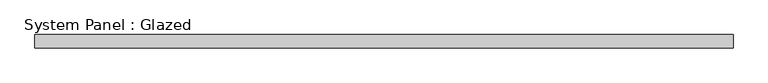
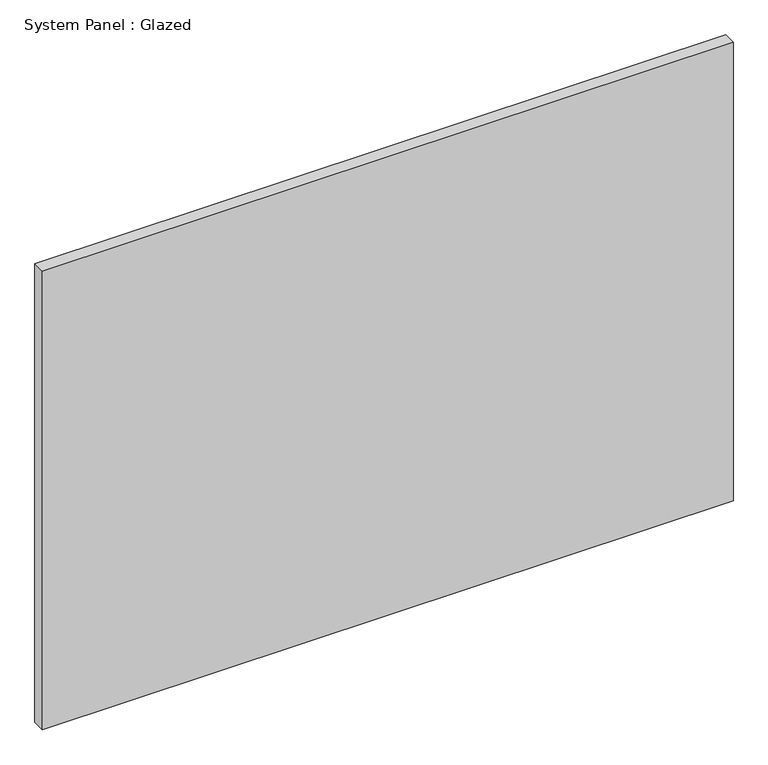
"""IFC4 building model written with IfcOpenShell, lengths in millimetres: plate geometry, System Panel : Glazed."""

from ifc_helpers import new_model, si_unit, origin, origin_with_axes, place, context, project, spatial, polyline, outline, extrude, source, transform, mapped, element, save


def system_panel_glazed_dc01897a(model_context):
    return source(origin(), model_context, "Body", "SweptSolid", [
        extrude(outline(polyline([(660.8, 24.5), (-660.8, 24.5), (-660.8, 49.5), (660.8, 49.5), (660.8, 24.5)])), origin_with_axes(), (0.0, 0.0, 1.0), 927.5595785),
    ])


if __name__ == "__main__":
    model = new_model("IFC4")
    model_context = context("Model", 3, world=origin())
    ifc_project = project(units=[si_unit("LENGTHUNIT", "METRE", prefix="MILLI")], contexts=[model_context])
    site = spatial("IfcSite", under=ifc_project)
    building = spatial("IfcBuilding", under=site)
    placement = place(None, origin())
    system_panel_glazed_shape = system_panel_glazed_dc01897a(model_context)
    element("IfcPlate", 1, ObjectType="System Panel : Glazed", at=placement, inside=building, context=model_context, shape_type="MappedRepresentation", body=[
        mapped(system_panel_glazed_shape, transform((0.0, 0.0, 0.0), x_axis=(1.0, 0.0, 0.0), y_axis=(0.0, 1.0, 0.0), z_axis=(0.0, 0.0, 1.0))),
    ])
    save(model, "model.ifc")

# Revit data of these elements
# Type "System Panel : Glazed"
#   Construction Type Id = "GSP4R"
#   Analytic Construction = "1/8 in Pilkington single glazing"
#   Visual Light Transmittance = 0.9
#   Solar Heat Gain Coefficient = 0.86
#   Heat Transfer Coefficient (U) = 6.7069 W/(m²·K)
# Element 1 (IfcPlate, "System Panel : Glazed")
#   Materials on its faces: "Glass"
# Materials
#   "Glass": class "Glass", colour RGB 0 128 192, transparency 0.9, Description = "Soda Lime Glass", Cost = 0
